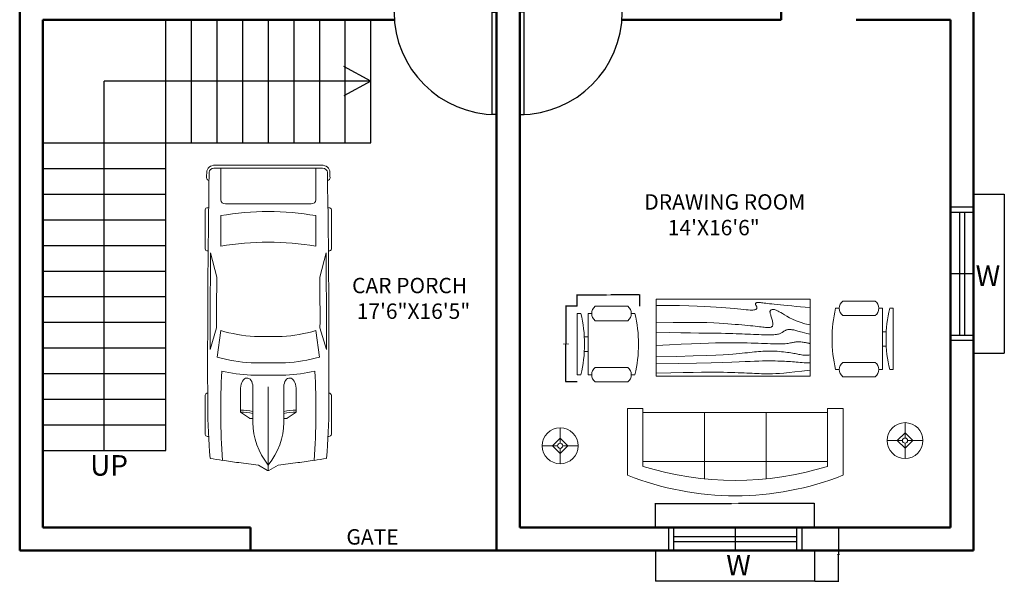
# Model space of a CAD drawing. Units: inches. Extents: x -8 to 1354, y -679 to 94.
# Tile 1 of 6: x 4 to 388, y -648 to -429. Entities that reach past the tile are written whole.
import ezdxf

# ---------------------------------------------------------------- set-up
doc = ezdxf.new("R2010")
doc.units = ezdxf.units.IN
doc.header["$MEASUREMENT"] = 0
for name, color, linetype, lineweight in [('A-ANNO-DIMS', 2, 'Continuous', 18), ('A-ANNO-TEXT', 7, 'Continuous', 25), ('A-AREA-IDEN', 7, 'Continuous', 25), ('A-DOOR', 3, 'Continuous', 25), ('A-FLOR-STRS', 2, 'Continuous', 25), ('A-FURN', 8, 'Continuous', 18), ('A-GLAZ', 4, 'Continuous', 25), ('A-SITE-VEHC', 9, 'Continuous', 13), ('A-WALL', 1, 'Continuous', 50)]:
    doc.layers.add(name, color=color, linetype=linetype, lineweight=lineweight)
doc.styles.get("Standard").update_dxf_attribs({"font": 'arial.ttf'})
doc.dimstyles.get("Standard").update_dxf_attribs({"dimtxt": 0.18, "dimasz": 0.18, "dimexe": 0.18, "dimexo": 0.0625, "dimgap": 0.09, "dimtad": 0, "dimtih": 1, "dimtoh": 1, "dimdec": 1, "dimzin": 0, "dimdsep": 46, "dimlunit": 4, "dimtxsty": 'Standard', "dimcen": 0.09, "dimclrd": 2, "dimclre": 3, "dimclrt": 6, "dimadec": 0, "dimazin": 0, "dimtfac": 1, "dimtdec": 1, "dimtofl": 0, "dimtmove": 0, "dimatfit": 3, "dimfxl": 1, "dimtfill": 2, "dimtfillclr": 4, "dimtolj": 1, "dimtzin": 0, "dimarcsym": 0})

# ---------------------------------------------------------------- blocks, each defined once
blk = doc.blocks.new('*U5')
for p, q in [((-40, 0), (-40, 6)), ((0, 0), (0, 6))]:
    blk.add_line(p, q)
blk.add_lwpolyline([(0, 0), (0, -40), (-1.75, -40), (-1.75, 0)], close=True)
blk.add_arc((0, 0), 40, 180, 270)
blk = doc.blocks.new('*U2')
for p, q in [((0, 0), (0, 6)), ((40, 0), (40, 6))]:
    blk.add_line(p, q)
blk.add_lwpolyline([(0, 0), (0, -40), (1.75, -40), (1.75, 0)], close=True)
blk.add_arc((0, 0), 40, 270, 0)
blk = doc.blocks.new('*U9')
for p, q in [((21.1, 37.41), (21.1, 36.83)), ((46.55, 38.89), (22.35, 38.89)), ((47.8, 37.39), (47.8, 37.41)), ((135.45, 37.07), (135.45, 37.41)), ((136.7, 38.89), (160.9, 38.89)), ((162.15, 37.41), (162.15, 36.77)), ((70.03, 31.54), (86.41, 29.35)), ((87.99, 31.87), (74.76, 35.92)), ((134.31, 35.6), (119.29, 31.78)), ((186.47, -33.5), (186.47, 33.5)), ((188.4, -32.76), (188.4, 32.76)), ((138.42, 29.35), (157.25, 29.35)), ((164.52, 26.39), (164.52, -26.39)), ((186.47, 29.35), (167.01, 29.35)), ((32.27, 11.63), (36.13, 17.17)), ((36.13, 17.17), (50.94, 17.17)), ((3.27, 6.13), (0.1, 0.41)), ((29.77, 9.51), (51.68, 9.51)), ((32.12, 9.51), (32.12, 11.15)), ((58.92, -10.77), (58.92, 10.77)), ((66.55, -10.53), (66.55, 10.53)), ((82.74, 8.5), (82.74, -8.5)), ((186.47, -10.53), (186.47, 10.53)), ((0, 0), (51.68, 0)), ((0.1, -0.41), (3.27, -6.13)), ((29.77, -9.51), (51.68, -9.51)), ((32.12, -9.51), (32.12, -11.15)), ((32.27, -11.63), (36.13, -17.17)), ((36.13, -17.17), (50.94, -17.17)), ((86.41, -29.35), (70.03, -31.54)), ((157.25, -29.35), (138.42, -29.35)), ((167.01, -29.35), (186.47, -29.35)), ((87.99, -31.87), (74.76, -35.92)), ((134.31, -35.6), (119.29, -31.78)), ((21.1, -37.41), (21.1, -36.83)), ((46.55, -38.89), (22.35, -38.89)), ((47.8, -37.39), (47.8, -37.41)), ((135.45, -37.07), (135.45, -37.41)), ((136.7, -38.89), (160.9, -38.89)), ((162.15, -37.41), (162.15, -36.77))]:
    blk.add_line(p, q)
for centre, major_axis, ratio, start_param, end_param in [((41.19, -490.86), (0, 528.23), 0.842304, 0.00281, 0.075598), ((22.35, 37.41), (0, -1.48), 0.842304, 3.141593, 4.712389), ((64.48, -10555.62), (0, 10593.03), 0.842304, -0.013397, 0.002797), ((46.55, 37.41), (0, 1.48), 0.842304, -1.570796, 0), ((136.7, 37.41), (0, -1.48), 0.842304, 3.141593, 4.712389), ((160.9, 37.41), (0, 1.48), 0.842304, -1.570796, 0), ((180.63, 35.84), (0, 2.22), 0.842304, -0.013017, 1.249894), ((64.48, -10556.36), (0, 10595.31), 0.842304, -0.013397, -0.013017), ((183.98, 33.5), (0, -2.96), 0.842304, 1.570796, 3.128196), ((183.98, 32.76), (0, -5.25), 0.842304, 1.570796, 3.128196), ((266.03, -27.52), (0, 313.31), 0.842304, 1.367076, 1.39176), ((135.29, 5.39), (0, 81.77), 0.842304, 1.245306, 1.50788), ((64.48, -10555.62), (0, -10591.55), 0.842304, 3.133765, 3.140441), ((95.79, -3666.35), (0, -3698.24), 0.842304, 3.134049, 3.144098), ((259.18, -27.52), (0, -305.3), 0.842304, 4.528606, 4.561838), ((37.47, -593.96), (0, -623.33), 0.842304, 3.096046, 3.200911), ((134.4, 5.39), (0, -89.78), 0.842304, 4.449482, 4.652344), ((149.6, 2.8), (0, -79.58), 0.842304, 4.372215, 4.640744), ((17.08, 0), (0, 147.02), 0.842304, 4.511394, 4.913384), ((35.91, 0), (0, 147.02), 0.842304, 4.511394, 4.913384), ((167.01, 26.39), (0, 2.96), 0.842304, 0, 1.570796), ((-204.49, 52.4), (0, -250.96), 0.842304, 1.385369, 1.434372), ((13.04, 17.01), (0, 27.42), 0.842304, 4.435146, 4.718221), ((14.2, 17.01), (0, 27.42), 0.842304, 4.435146, 4.718221), ((50.79, 13.34), (6.34, -0.36), 0.603834, -1.395552, 1.581315), ((29.77, -46.66), (0, 56.17), 0.842304, 0, 0.590319), ((32.75, 11.15), (0, 0.74), 0.842304, 0.879714, 1.570796), ((0.62, 0), (0, -0.74), 0.842304, 4.131459, 5.293319), ((29.77, 46.66), (0, 56.17), 0.842304, 2.551274, 3.141593), ((-204.49, -52.4), (0, 250.96), 0.842304, -1.434372, -1.385369), ((32.75, -11.15), (0, -0.74), 0.842304, 4.712389, 5.403472), ((13.04, -17.01), (0, -27.42), 0.842304, 1.564964, 1.848039), ((14.2, -17.01), (0, -27.42), 0.842304, 1.564964, 1.848039), ((134.4, -5.39), (0, -89.78), 0.842304, -1.510751, -1.307889), ((135.29, -5.39), (0, -81.77), 0.842304, -1.50788, -1.245306), ((149.6, -2.8), (0, -79.58), 0.842304, -1.499151, -1.230623), ((259.18, 27.52), (0, 305.3), 0.842304, 1.721348, 1.754579), ((266.03, 27.52), (0, 313.31), 0.842304, 1.749832, 1.774517), ((37.47, 593.96), (0, -623.33), 0.842304, -0.059319, 0.045547), ((167.01, -26.39), (0, -2.96), 0.842304, 4.712389, 6.283185), ((41.19, 490.86), (0, -528.23), 0.842304, -0.075598, -0.00281), ((64.48, 10555.62), (0, -10591.55), 0.842304, 0.001152, 0.007828), ((95.79, 3666.35), (0, -3698.24), 0.842304, -0.002505, 0.007544), ((183.98, -33.5), (0, 2.96), 0.842304, 3.15499, 4.712389), ((183.98, -32.76), (0, -5.25), 0.842304, 0.013397, 1.570796), ((22.35, -37.41), (0, 1.48), 0.842304, 1.570796, 3.141593), ((64.48, 10555.62), (0, 10593.03), 0.842304, 3.138796, 3.15499), ((46.55, -37.41), (0, -1.48), 0.842304, 0, 1.570796), ((136.7, -37.41), (0, -1.48), 0.842304, -1.570796, 0), ((160.9, -37.41), (0, 1.48), 0.842304, 3.141593, 4.712389), ((180.63, -35.84), (0, -2.22), 0.842304, -1.249894, 0.013017), ((64.48, 10556.36), (0, 10595.31), 0.842304, 3.15461, 3.15499)]:
    blk.add_ellipse(centre, major_axis=major_axis, ratio=ratio, start_param=start_param, end_param=end_param)
at = {"extrusion": (0, 0, -1)}
blk.add_ellipse((50.79, -13.34), major_axis=(6.34, 0.36), ratio=0.603834, start_param=-1.395552, end_param=1.581315, dxfattribs=at)
blk = doc.blocks.new('Sofa - Roundback 7 ft.')
for p, q in [((-12.00002, -32.4421), (-12.00003, -6.5971)), ((11.99997, -32.4421), (11.99998, -6.5971)), ((-36.000027, -34), (-36.000027, -11.4696)), ((35.99998, -34), (35.99998, -11.4696)), ((-35.999844, -13.3819), (35.9998, -13.3819)), ((-36.000027, -32.4421), (35.99998, -32.4421))]:
    blk.add_line(p, q)
for points in [[(-36.000027, -34), (-42.000027, -34), (-42.000027, -8)], [(41.99998, -8), (41.99998, -34), (35.99998, -34)]]:
    blk.add_lwpolyline(points)
for centre, radius, start, end in [((0, -114.25), 114.25, 68.43141, 111.5686), ((-0.00001, -127.1968), 121.1968, 72.72033, 107.2797)]:
    blk.add_arc(centre, radius, start, end)
blk = doc.blocks.new('Table - Rectangular Woodgrain 60 x 30 in.')
for p, q in [((0, 0), (0, -30)), ((60, 0), (0, 0)), ((60, -30), (60, 0)), ((0, -30), (60, -30))]:
    blk.add_line(p, q)
for points in [[(0, -2.4), (4.8155, -2.418), (9.0302, -2.4688), (12.709, -2.5477), (15.9167, -2.65), (18.7181, -2.7711), (21.1781, -2.9063), (23.3616, -3.0508), (25.3333, -3.2), (27.1477, -3.3495), (28.8172, -3.4958), (30.3437, -3.636), (31.7291, -3.7667), (32.9756, -3.8849), (34.0849, -3.9875), (35.059, -4.0714), (35.9, -4.1334), (36.6114, -4.1711), (37.2041, -4.1854), (37.6906, -4.1779), (38.0833, -4.15), (38.3948, -4.1034), (38.6375, -4.0396), (38.8239, -3.9602), (38.9666, -3.8667), (39.0764, -3.7608), (39.1573, -3.6448), (39.2116, -3.521), (39.2416, -3.3917), (39.2498, -3.2593), (39.2385, -3.1261), (39.21, -2.9944), (39.1666, -2.8667), (39.111, -2.7447), (39.0468, -2.6281), (38.978, -2.5163), (38.9083, -2.4083), (38.8418, -2.3035), (38.7823, -2.201), (38.7337, -2.1001), (38.7, -2), (38.6844, -1.9003), (38.6875, -1.8021), (38.7094, -1.707), (38.75, -1.6167), (38.8094, -1.5326), (38.8875, -1.4563), (38.9844, -1.3893), (39.1, -1.3333), (39.2351, -1.2896), (39.3937, -1.2583), (39.5804, -1.2396), (39.8, -1.2333), (40.057, -1.2396), (40.3562, -1.2583), (40.7023, -1.2896), (41.1, -1.3333), (41.5547, -1.3895), (42.0755, -1.4573), (42.6721, -1.5361), (43.3542, -1.625), (44.1316, -1.7233), (45.014, -1.8302), (46.0114, -1.9449), (47.1333, -2.0667), (48.3862, -2.1947), (49.7625, -2.3281), (51.2513, -2.4663), (52.8416, -2.6083), (54.5226, -2.7535), (56.2833, -2.9011), (58.1127, -3.0501), (60, -3.2)], [(0, -9.2), (6.5759, -9.0858), (11.9385, -9.0365), (16.2527, -9.0418), (19.6833, -9.0917), (22.3952, -9.1759), (24.5531, -9.2844), (26.322, -9.4069), (27.8666, -9.5333), (29.3241, -9.6553), (30.7203, -9.7719), (32.0532, -9.8837), (33.3208, -9.9917), (34.5213, -10.0965), (35.6526, -10.199), (36.7128, -10.2999), (37.7, -10.4), (38.6129, -10.4996), (39.4531, -10.5969), (40.223, -10.6895), (40.925, -10.775), (41.5613, -10.8512), (42.1344, -10.9156), (42.6465, -10.966), (43.1, -11), (43.4976, -11.0158), (43.8437, -11.0136), (44.143, -10.9942), (44.4, -10.9583), (44.6195, -10.9069), (44.8062, -10.8406), (44.9648, -10.7603), (45.1, -10.6667), (45.2155, -10.5598), (45.3114, -10.4365), (45.3871, -10.2929), (45.4416, -10.125), (45.4743, -9.929), (45.4844, -9.7011), (45.4709, -9.4371), (45.4333, -9.1333), (45.3716, -8.7883), (45.2896, -8.4104), (45.1919, -8.0107), (45.0833, -7.6), (44.9685, -7.1893), (44.8521, -6.7896), (44.7388, -6.4117), (44.6333, -6.0667), (44.54, -5.7628), (44.4614, -5.4979), (44.4001, -5.2675), (44.3583, -5.0667), (44.3384, -4.8909), (44.3427, -4.7354), (44.3736, -4.5956), (44.4333, -4.4667), (44.5236, -4.3453), (44.6427, -4.2333), (44.7884, -4.1339), (44.9583, -4.05), (45.1501, -3.9849), (45.3614, -3.9417), (45.59, -3.9234), (45.8333, -3.9333), (46.0915, -3.9749), (46.3734, -4.0531), (46.6906, -4.1736), (47.0542, -4.3417), (47.4756, -4.5629), (47.9661, -4.8427), (48.5372, -5.1866), (49.2, -5.6), (49.9676, -6.0844), (50.8594, -6.625), (51.8965, -7.2031), (53.1, -7.8), (54.491, -8.3969), (56.0906, -8.975), (57.9199, -9.5156), (60, -10)], [(0, -12.8), (5.1847, -12.9322), (9.6213, -13.0323), (13.3963, -13.1059), (16.5958, -13.1583), (19.3063, -13.1952), (21.614, -13.2219), (23.6054, -13.2439), (25.3666, -13.2667), (26.9728, -13.2947), (28.4531, -13.3281), (29.8256, -13.3663), (31.1083, -13.4083), (32.3191, -13.4535), (33.476, -13.501), (34.597, -13.5501), (35.7, -13.6), (36.7984, -13.6497), (37.8875, -13.6979), (38.9578, -13.743), (40, -13.7833), (41.0047, -13.8174), (41.9625, -13.8438), (42.864, -13.8607), (43.7, -13.8667), (44.4631, -13.8604), (45.1552, -13.8417), (45.7801, -13.8104), (46.3416, -13.7667), (46.8439, -13.7104), (47.2906, -13.6417), (47.6858, -13.5604), (48.0333, -13.4667), (48.3375, -13.3608), (48.6042, -13.2448), (48.8396, -13.121), (49.05, -12.9917), (49.2417, -12.8593), (49.4208, -12.7261), (49.5937, -12.5944), (49.7667, -12.4667), (49.9452, -12.3451), (50.1323, -12.2313), (50.3303, -12.1268), (50.5416, -12.0333), (50.7686, -11.9524), (51.0135, -11.8854), (51.2788, -11.8341), (51.5666, -11.8), (51.8785, -11.7843), (52.2116, -11.7865), (52.562, -11.8059), (52.926, -11.8417), (53.2998, -11.8931), (53.6795, -11.9594), (54.0614, -12.0397), (54.4416, -12.1333), (54.8223, -12.2401), (55.2293, -12.3625), (55.6942, -12.5037), (56.2489, -12.6667), (56.9251, -12.8547), (57.7545, -13.0708), (58.7689, -13.3182), (60, -13.6)], [(0, -18), (5.124, -17.7273), (9.6609, -17.5057), (13.6705, -17.3303), (17.2125, -17.1958), (20.3467, -17.0973), (23.1328, -17.0297), (25.6307, -16.9878), (27.9, -16.9667), (29.9928, -16.9617), (31.9302, -16.9703), (33.7254, -16.9907), (35.3917, -17.0208), (36.9423, -17.0588), (38.3906, -17.1026), (39.7499, -17.1503), (41.0333, -17.2), (42.2519, -17.2496), (43.4073, -17.2969), (44.4986, -17.3395), (45.525, -17.375), (46.4858, -17.4012), (47.3802, -17.4156), (48.2074, -17.416), (48.9667, -17.4), (49.6583, -17.3662), (50.2872, -17.3167), (50.8595, -17.2547), (51.3812, -17.1833), (51.8584, -17.1057), (52.2971, -17.025), (52.7034, -16.9443), (53.0833, -16.8667), (53.443, -16.7951), (53.789, -16.7313), (54.128, -16.6768), (54.4666, -16.6334), (54.8115, -16.6024), (55.1693, -16.5854), (55.5465, -16.5841), (55.95, -16.6), (56.3828, -16.6337), (56.8346, -16.6823), (57.2915, -16.7418), (57.7396, -16.8084), (58.165, -16.878), (58.5539, -16.9469), (58.8924, -17.0111), (59.1666, -17.0667), (59.3679, -17.1107), (59.5078, -17.1438), (59.6032, -17.1675), (59.6708, -17.1833), (59.7275, -17.193), (59.7901, -17.1979), (59.8753, -17.1998), (60, -17.2)], [(0, -22.4), (8.0098, -22.2501), (14.4094, -22.1011), (19.4168, -21.9535), (23.25, -21.8083), (26.1269, -21.6663), (28.2656, -21.5281), (29.884, -21.3947), (31.2, -21.2667), (32.3967, -21.1448), (33.5172, -21.0292), (34.5697, -20.9198), (35.5625, -20.8167), (36.5037, -20.7198), (37.4015, -20.6292), (38.2642, -20.5448), (39.1, -20.4667), (39.9164, -20.3951), (40.7187, -20.3313), (41.5117, -20.2768), (42.3, -20.2333), (43.0883, -20.2024), (43.8812, -20.1854), (44.6836, -20.1841), (45.5, -20.2), (46.3328, -20.234), (47.1747, -20.2844), (48.0163, -20.3488), (48.8479, -20.425), (49.66, -20.5106), (50.4429, -20.6031), (51.1872, -20.7004), (51.8833, -20.8), (52.5246, -20.8999), (53.1166, -20.9995), (53.6681, -21.0983), (54.1875, -21.1958), (54.6834, -21.2919), (55.1646, -21.3859), (55.6394, -21.4777), (56.1167, -21.5667), (56.6028, -21.6515), (57.0961, -21.7266), (57.5929, -21.7852), (58.0896, -21.8208), (58.5823, -21.8268), (59.0674, -21.7964), (59.5412, -21.723), (60, -21.6)], [(0, -25.2), (8.6355, -25.0504), (15.7026, -24.9031), (21.4049, -24.7606), (25.9458, -24.625), (29.529, -24.4988), (32.3578, -24.3844), (34.6359, -24.284), (36.5667, -24.2), (38.3213, -24.1341), (39.9417, -24.0854), (41.437, -24.0523), (42.8167, -24.0333), (44.0901, -24.0268), (45.2667, -24.0313), (46.3557, -24.0451), (47.3667, -24.0667), (48.309, -24.0947), (49.1928, -24.1287), (50.0284, -24.168), (50.826, -24.2125), (51.5959, -24.2617), (52.3483, -24.3151), (53.0935, -24.3725), (53.8417, -24.4334), (54.6009, -24.497), (55.3699, -24.561), (56.1454, -24.6226), (56.9239, -24.6792), (57.7021, -24.7279), (58.4764, -24.7662), (59.2435, -24.7911), (60, -24.8)], [(0, -28.8), (5.6867, -28.6681), (10.45, -28.5698), (14.407, -28.5012), (17.675, -28.4584), (20.3711, -28.4374), (22.6125, -28.4344), (24.5164, -28.4455), (26.2, -28.4667), (27.762, -28.4947), (29.2276, -28.5281), (30.6033, -28.5663), (31.8958, -28.6084), (33.1118, -28.6535), (34.2578, -28.7011), (35.3405, -28.7501), (36.3666, -28.8), (37.3443, -28.8497), (38.288, -28.8974), (39.2137, -28.9412), (40.1375, -28.9792), (41.0753, -29.0093), (42.0432, -29.0297), (43.0572, -29.0384), (44.1333, -29.0333), (45.2936, -29.0114), (46.5843, -28.9641), (48.0579, -28.8816), (49.7666, -28.7542), (51.7629, -28.5721), (54.0989, -28.3255), (56.8272, -28.0048), (60, -27.6)]]:
    blk.add_lwpolyline(points)
blk = doc.blocks.new('Lamp - Table')
for p, q in [((0, 7), (0, 1)), ((-1, 0), (-7, 0)), ((0, 3), (-3, 0)), ((-3, 0), (0, -3)), ((3, 0), (0, 3)), ((0, -3), (3, 0)), ((1, 0), (7, 0)), ((0, -1), (0, -7))]:
    blk.add_line(p, q)
for radius in [7, 1]:
    blk.add_circle((0, 0), radius)
blk = doc.blocks.new('Chair - Desk')
for p, q in [((-8.5, 0), (-8.5, -1)), ((-8.5, 0), (8.5, 0)), ((8.5, 0), (8.5, -1)), ((-2, -3), (-2, -1.9355)), ((2, -1.9576), (2, -3)), ((-10.5, -5), (-10.5, -14)), ((-8.5, -3), (-8.5, -4)), ((-8.5, -3), (8.5, -3)), ((-6.5, -14), (-6.5, -5)), ((6.5, -5), (6.5, -14)), ((8.5, -3), (8.5, -4)), ((10.5, -14), (10.5, -5)), ((-8.5, -15), (-8.5, -16)), ((8.5, -15), (8.5, -16))]:
    blk.add_line(p, q)
for centre, radius, start, end in [((0, 34.625), 36.625, 256.5803, 283.4197), ((-8.5, -6.5), 2.5, 36.8699, 143.1301), ((8.5, -6.5), 2.5, 36.8699, 143.1301), ((-8.5, -12.5), 2.5, 216.8699, 323.1301), ((0, 19.625), 36.625, 256.5803, 283.4197), ((8.5, -12.5), 2.5, 216.8699, 323.1301)]:
    blk.add_arc(centre, radius, start, end)
blk = doc.blocks.new('WIN-W')
at = {"ltscale": 2}
for p, q in [((12, 62), (0, 62)), ((0, 0), (0, 62)), ((12, 57), (12, 62)), ((12, 5), (12, 0)), ((12, 0), (0, 0))]:
    blk.add_line(p, q, dxfattribs=at)
for p, q in [((21, 57), (12, 57)), ((21, 5), (12, 5))]:
    blk.add_line(p, q)
blk = doc.blocks.new('*D81')
at = {"layer": 'A-ANNO-DIMS', "color": 3, "lineweight": -2, "transparency": 16777216}
for p, q in [((252.16, -626.76), (252.16, -617.35)), ((314.16, -626.76), (314.16, -617.35))]:
    blk.add_line(p, q, dxfattribs=at)
at = {"layer": 'A-ANNO-DIMS', "color": 2, "lineweight": -2, "transparency": 16777216}
for p, q in [((252.34, -617.53), (281.78, -617.53)), ((313.98, -617.53), (284.54, -617.53))]:
    blk.add_line(p, q, dxfattribs=at)
at = {"layer": 'A-ANNO-DIMS', "color": 2, "transparency": 16777216}
for points in [[(252.34, -617.5), (252.34, -617.56), (252.16, -617.53)], [(313.98, -617.5), (313.98, -617.56), (314.16, -617.53)]]:
    blk.add_solid(points, dxfattribs=at)
at = {"layer": 'Defpoints', "color": 0, "transparency": 16777216}
for p in [(252.16, -617.53), (252.16, -626.83), (314.16, -626.83)]:
    blk.add_point(p, dxfattribs=at)
at = {"layer": 'A-ANNO-DIMS', "color": 6, "transparency": 16777216, "insert": (283.16, -617.53), "char_height": 0.18, "attachment_point": 5, "bg_fill": 1, "box_fill_scale": 1.25, "bg_fill_color": 4, "bg_fill_transparency": 0}
blk.add_mtext('\\A1;WINDOW W 5\'-2" TYP.', dxfattribs=at)
blk = doc.blocks.new('*D82')
at = {"layer": 'A-ANNO-DIMS', "color": 3, "lineweight": -2, "transparency": 16777216}
for p, q in [((314.22, -626.83), (323.64, -626.83)), ((314.22, -647.83), (323.64, -647.83))]:
    blk.add_line(p, q, dxfattribs=at)
at = {"layer": 'A-ANNO-DIMS', "color": 2, "lineweight": -2, "transparency": 16777216}
for p, q in [((323.46, -627.01), (323.46, -637.14)), ((323.46, -647.65), (323.46, -637.51))]:
    blk.add_line(p, q, dxfattribs=at)
at = {"layer": 'A-ANNO-DIMS', "color": 2, "transparency": 16777216}
for points in [[(323.43, -627.01), (323.49, -627.01), (323.46, -626.83)], [(323.43, -647.65), (323.49, -647.65), (323.46, -647.83)]]:
    blk.add_solid(points, dxfattribs=at)
at = {"layer": 'Defpoints', "color": 0, "transparency": 16777216}
for p in [(314.16, -626.83), (323.46, -626.83), (314.16, -647.83)]:
    blk.add_point(p, dxfattribs=at)
at = {"layer": 'A-ANNO-DIMS', "color": 6, "transparency": 16777216, "insert": (323.46, -637.33), "char_height": 0.18, "attachment_point": 5, "bg_fill": 1, "box_fill_scale": 1.25, "bg_fill_color": 4, "bg_fill_transparency": 0}
blk.add_mtext('\\A1;1\'-9" TYP.', dxfattribs=at)
blk = doc.blocks.new('*D87')
at = {"layer": 'A-ANNO-DIMS', "color": 3, "lineweight": -2, "transparency": 16777216}
for p, q in [((221.57, -540.59), (217.03, -540.59)), ((221.57, -570.08), (217.03, -570.08))]:
    blk.add_line(p, q, dxfattribs=at)
at = {"layer": 'A-ANNO-DIMS', "color": 2, "lineweight": -2, "transparency": 16777216}
for p, q in [((217.21, -540.77), (217.21, -555.15)), ((217.21, -569.9), (217.21, -555.52))]:
    blk.add_line(p, q, dxfattribs=at)
at = {"layer": 'A-ANNO-DIMS', "color": 2, "transparency": 16777216}
for points in [[(217.18, -540.77), (217.24, -540.77), (217.21, -540.59)], [(217.18, -569.9), (217.24, -569.9), (217.21, -570.08)]]:
    blk.add_solid(points, dxfattribs=at)
at = {"layer": 'Defpoints', "color": 0, "transparency": 16777216}
for p in [(221.63, -540.59), (217.21, -570.08), (221.63, -570.08)]:
    blk.add_point(p, dxfattribs=at)
at = {"layer": 'A-ANNO-DIMS', "color": 6, "transparency": 16777216, "insert": (217.21, -555.34), "char_height": 0.18, "attachment_point": 5, "bg_fill": 1, "box_fill_scale": 1.25, "bg_fill_color": 4, "bg_fill_transparency": 0}
blk.add_mtext('\\A1;CHAIR 2\'-5 1/2" TYP.', dxfattribs=at)
blk = doc.blocks.new('*D88')
at = {"layer": 'A-ANNO-DIMS', "color": 3, "lineweight": -2, "transparency": 16777216}
for p, q in [((221.63, -540.52), (221.63, -535.98)), ((245.98, -540.52), (245.98, -535.98))]:
    blk.add_line(p, q, dxfattribs=at)
at = {"layer": 'A-ANNO-DIMS', "color": 2, "lineweight": -2, "transparency": 16777216}
for p, q in [((221.81, -536.16), (232.96, -536.16)), ((245.8, -536.16), (234.66, -536.16))]:
    blk.add_line(p, q, dxfattribs=at)
at = {"layer": 'A-ANNO-DIMS', "color": 2, "transparency": 16777216}
for points in [[(221.81, -536.13), (221.81, -536.19), (221.63, -536.16)], [(245.8, -536.13), (245.8, -536.19), (245.98, -536.16)]]:
    blk.add_solid(points, dxfattribs=at)
at = {"layer": 'Defpoints', "color": 0, "transparency": 16777216}
for p in [(221.63, -536.16), (221.63, -540.59), (245.98, -540.59)]:
    blk.add_point(p, dxfattribs=at)
at = {"layer": 'A-ANNO-DIMS', "color": 6, "transparency": 16777216, "insert": (233.81, -536.16), "char_height": 0.18, "attachment_point": 5, "bg_fill": 1, "box_fill_scale": 1.25, "bg_fill_color": 4, "bg_fill_transparency": 0}
blk.add_mtext('\\A1;2\'-0 1/2" TYP.', dxfattribs=at)

msp = doc.modelspace()

# ---------------------------------------------------------------- linework, layer by layer
at = {"layer": 'A-FLOR-STRS'}
for p, q in [((61.16, -476.83), (61.16, -428.83)), ((71.16, -476.83), (71.16, -428.83)), ((81.16, -476.83), (81.16, -428.83)), ((91.16, -476.83), (91.16, -428.83)), ((101.16, -476.83), (101.16, -428.83)), ((111.16, -476.83), (111.16, -428.83)), ((121.16, -476.83), (121.16, -428.83)), ((131.16, -476.83), (131.16, -428.83)), ((141.16, -476.83), (141.16, -428.83)), ((141.16, -452.83), (130.56, -447.1)), ((141.16, -452.83), (37.16, -452.83)), ((37.16, -596.83), (37.16, -452.83)), ((141.16, -452.83), (130.56, -458.55)), ((13.16, -476.83), (61.16, -476.83)), ((61.16, -596.83), (61.16, -476.83)), ((61.16, -476.83), (141.16, -476.83)), ((13.16, -486.83), (61.16, -486.83)), ((13.16, -496.83), (61.16, -496.83)), ((13.16, -506.83), (61.16, -506.83)), ((13.16, -516.83), (61.16, -516.83)), ((13.16, -526.83), (61.16, -526.83)), ((13.16, -536.83), (61.16, -536.83)), ((13.16, -546.83), (61.16, -546.83)), ((13.16, -556.83), (61.16, -556.83)), ((13.16, -566.83), (61.16, -566.83)), ((13.16, -576.83), (61.16, -576.83)), ((13.16, -586.83), (61.16, -586.83)), ((13.16, -596.83), (61.16, -596.83))]:
    msp.add_line(p, q, dxfattribs=at)
at = {"layer": 'A-GLAZ'}
for p, q in [((367.16, -503.83), (376.16, -503.83)), ((370.66, -503.83), (370.66, -551.83)), ((372.66, -503.83), (372.66, -551.83)), ((367.16, -527.83), (376.16, -527.83)), ((367.16, -551.83), (376.16, -551.83)), ((259.16, -626.83), (259.16, -635.83)), ((283.16, -626.83), (283.16, -635.83)), ((307.16, -626.83), (307.16, -635.83)), ((259.16, -630.33), (307.16, -630.33)), ((259.16, -632.33), (307.16, -632.33))]:
    msp.add_line(p, q, dxfattribs=at)
at = {"layer": 'A-WALL'}
for p, q in [((4.16, -59.83), (4.16, -635.83)), ((301.16, -428.83), (301.16, -341.83)), ((376.16, -341.83), (376.16, -428.83)), ((190.16, -635.72), (190.16, -419.83)), ((199.16, -626.83), (199.16, -419.83)), ((13.16, -428.83), (13.16, -626.83)), ((150.27, -428.83), (13.16, -428.83)), ((61.16, -428.83), (13.16, -428.83)), ((301.16, -428.83), (239.05, -428.83)), ((301.16, -428.83), (250.16, -428.83)), ((367.16, -428.83), (330.42, -428.83)), ((367.16, -428.83), (330.42, -428.83)), ((367.16, -428.83), (367.16, -626.83)), ((376.16, -428.83), (376.16, -635.83)), ((94.16, -626.83), (13.16, -626.83)), ((94.16, -626.83), (94.16, -635.83)), ((367.16, -626.83), (199.16, -626.83)), ((94.16, -635.83), (4.16, -635.83)), ((94.16, -635.83), (190.16, -635.83)), ((376.16, -635.83), (190.16, -635.83))]:
    msp.add_line(p, q, dxfattribs=at)

# ---------------------------------------------------------------- block references
at = {"layer": 'A-DOOR'}
for name, p in [('*U5', (190.16, -425.83)), ('*U2', (199.16, -425.83))]:
    msp.add_blockref(name, p, dxfattribs=at)
at = {"layer": 'A-FURN', "yscale": 1.404642118538679, "zscale": 1.404642118538679}
for p, xscale, rotation in [((221.63, -555.34), -1.404642118538679, 90), ((344.86, -553.32), 1.404642118538679, 270)]:
    msp.add_blockref('Chair - Desk', p, dxfattribs=dict(at, xscale=xscale, rotation=rotation))
at = {"layer": 'A-FURN'}
for name, p in [('Table - Rectangular Woodgrain 60 x 30 in.', (252.43, -537.86)), ('Lamp - Table', (349.44, -592.96)), ('Lamp - Table', (214.94, -594.98))]:
    msp.add_blockref(name, p, dxfattribs=at)
at = {"layer": 'A-FURN', "rotation": 180}
msp.add_blockref('Sofa - Roundback 7 ft.', (283.25, -614.47), dxfattribs=at)
at = {"layer": 'A-GLAZ'}
for p, rotation in [((388.16, -496.83), 180), ((314.16, -647.83), 89.99999999999969)]:
    msp.add_blockref('WIN-W', p, dxfattribs=dict(at, rotation=rotation))
at = {"layer": 'A-SITE-VEHC', "xscale": 0.6323365212941213, "yscale": 0.6323365212941213, "zscale": 0.6323365212941213, "rotation": 90}
msp.add_blockref('*U9', (101.12, -604.67), dxfattribs=at)

# ---------------------------------------------------------------- texts
at = {"layer": 'A-ANNO-TEXT', "attachment_point": 1}
for s, insert, char_height in [('W', (376.98, -524.67), 8), ('UP', (31.63, -598.62), 8), ('GATE', (131.58, -627.51), 6), ('W', (279.71, -637.53), 8)]:
    msp.add_mtext_dynamic_manual_height_columns(s, width=71.0443, gutter_width=1, heights=[0], dxfattribs=dict(at, insert=insert, char_height=char_height))
at = {"layer": 'A-AREA-IDEN', "char_height": 6, "attachment_point": 1}
for s, insert in [('DRAWING ROOM\\P     14\'X16\'6"', (247.77, -496.89)), ('CAR PORCH\\P 17\'6"X16\'5"', (133.78, -529.49))]:
    msp.add_mtext_dynamic_manual_height_columns(s, width=71.0443, gutter_width=1, heights=[0], dxfattribs=dict(at, insert=insert))

# ---------------------------------------------------------------- dimensions: what is measured, and where the dimension line sits
at = {"layer": 'A-ANNO-DIMS'}
for base, p1, p2, angle, text, picture, middle in [((221.6321, -536.1617), (245.9793, -540.5864), (221.6321, -540.5864), 180, '<> TYP.', '*D88', (233.8057, -536.1617)), ((217.21, -570.08), (221.63, -540.59), (221.63, -570.08), 270, 'CHAIR <> TYP.', '*D87', (217.21, -555.34)), ((252.16, -617.53), (314.16, -626.83), (252.16, -626.83), 180, 'WINDOW W <> TYP.', '*D81', (283.16, -617.53)), ((323.46, -626.83), (314.16, -647.83), (314.16, -626.83), 90, '<> TYP.', '*D82', (323.46, -637.33))]:
    dim = msp.add_linear_dim(base=base, p1=p1, p2=p2, angle=angle, text=text, dimstyle='Standard', override={"dimdec": 1, "dimrnd": 0, "dimzin": 1, "dimlunit": 4, "dimfrac": 2}, dxfattribs=at)
    dim.commit()
    dim.dimension.update_dxf_attribs({"geometry": picture, "text_midpoint": middle})

doc.saveas('drawing.dxf')
